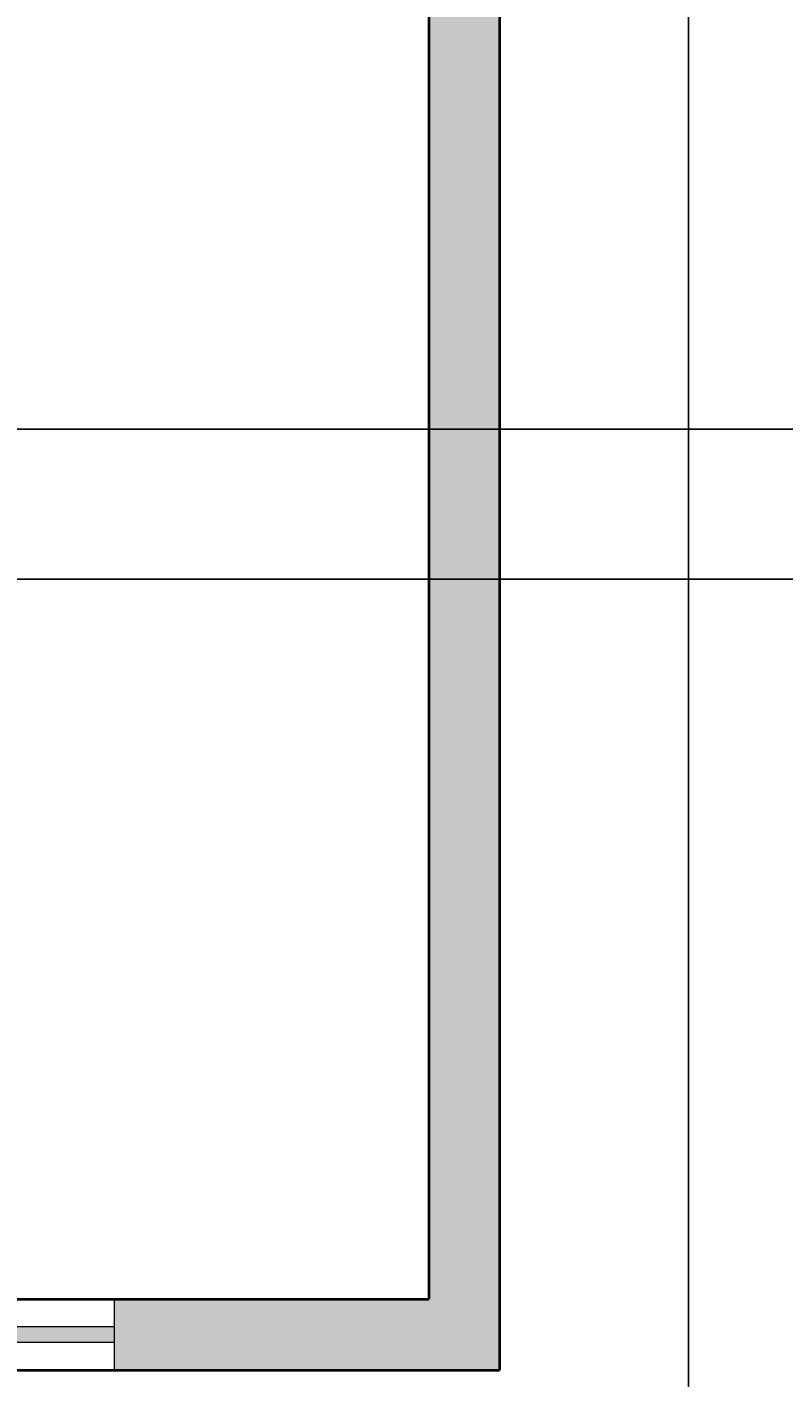
# Model space of a CAD drawing. Units: inches. Extents: x 2330 to 3943, y 1763 to 3461.
# Tile 8 of 40: x 2634 to 2730, y 2211 to 2383. Entities that reach past the tile are written whole.
import ezdxf

# ---------------------------------------------------------------- set-up
doc = ezdxf.new("R2010")
doc.units = ezdxf.units.IN
for name, color, linetype, lineweight in [('A-ANNO-DIMS', 2, 'Continuous', 18), ('A-GLAZ', 4, 'Continuous', 18), ('A-WALL', 7, 'Continuous', 40), ('A-WALL-PATT', 252, 'Continuous', 13)]:
    doc.layers.add(name, color=color, linetype=linetype, lineweight=lineweight)
doc.styles.get("Standard").update_dxf_attribs({"font": 'arial.ttf'})
doc.dimstyles.get("Standard").update_dxf_attribs({"dimtxt": 0.18, "dimasz": 0.18, "dimexe": 0.18, "dimexo": 0.0625, "dimgap": 0.09, "dimtad": 0, "dimtih": 1, "dimtoh": 1, "dimdec": 4, "dimzin": 0, "dimdsep": 46, "dimtxsty": 'Standard', "dimcen": 0.09, "dimadec": 0, "dimazin": 0, "dimtfac": 1, "dimtdec": 4, "dimtofl": 0, "dimtmove": 0, "dimatfit": 3, "dimfxl": 1, "dimtolj": 1, "dimtzin": 0, "dimarcsym": 0})

# ---------------------------------------------------------------- blocks, each defined once
blk = doc.blocks.new('WINDOW-120IN')
h = blk.add_hatch(color=256)
h.dxf.hatch_style = 1
h.paths.add_polyline_path([(120, 5.5), (0, 5.5), (0, 3.5), (120, 3.5)])
for p, q in [((0, 9), (0, 0)), ((120, 9), (120, 0)), ((120, 5.5), (0, 5.5)), ((120, 3.5), (0, 3.5))]:
    blk.add_line(p, q)
blk = doc.blocks.new('*D77')
at = {"layer": 'A-ANNO-DIMS', "color": 0, "lineweight": -2, "transparency": 16777216}
for p, q in [((2717.66, 2412.59), (2717.66, 1901.2)), ((2944.66, 2412.59), (2944.66, 1901.2)), ((2717.84, 1901.38), (2830.87, 1901.38)), ((2944.48, 1901.38), (2831.45, 1901.38))]:
    blk.add_line(p, q, dxfattribs=at)
at = {"layer": 'A-ANNO-DIMS', "color": 0, "transparency": 16777216}
for points in [[(2717.84, 1901.41), (2717.84, 1901.35), (2717.66, 1901.38)], [(2944.48, 1901.41), (2944.48, 1901.35), (2944.66, 1901.38)]]:
    blk.add_solid(points, dxfattribs=at)
at = {"layer": 'Defpoints', "color": 0, "transparency": 16777216}
for p in [(2717.66, 2412.65), (2944.66, 2412.65), (2944.66, 1901.38)]:
    blk.add_point(p, dxfattribs=at)
at = {"layer": 'A-ANNO-DIMS', "color": 0, "transparency": 16777216, "insert": (2831.16, 1901.38), "char_height": 0.18, "attachment_point": 5}
blk.add_mtext('\\A1;227', dxfattribs=at)
blk = doc.blocks.new('*D80')
at = {"layer": 'A-ANNO-DIMS', "color": 0, "lineweight": -2, "transparency": 16777216}
for p, q in [((3166.6, 2331.7), (2330.5, 2331.7)), ((2330.68, 2331.52), (2330.68, 2322.36)), ((2330.68, 2312.83), (2330.68, 2321.99)), ((3166.6, 2312.65), (2330.5, 2312.65))]:
    blk.add_line(p, q, dxfattribs=at)
at = {"layer": 'A-ANNO-DIMS', "color": 0, "transparency": 16777216}
for points in [[(2330.65, 2331.52), (2330.71, 2331.52), (2330.68, 2331.7)], [(2330.65, 2312.83), (2330.71, 2312.83), (2330.68, 2312.65)]]:
    blk.add_solid(points, dxfattribs=at)
at = {"layer": 'Defpoints', "color": 0, "transparency": 16777216}
for p in [(2330.68, 2331.7), (3166.66, 2331.7), (3166.66, 2312.65)]:
    blk.add_point(p, dxfattribs=at)
at = {"layer": 'A-ANNO-DIMS', "color": 0, "transparency": 16777216, "insert": (2330.68, 2322.18), "char_height": 0.18, "attachment_point": 5}
blk.add_mtext('\\A1;19.046', dxfattribs=at)

msp = doc.modelspace()

# ---------------------------------------------------------------- hatches: boundary and pattern name
at = {"layer": 'A-WALL-PATT'}
h = msp.add_hatch(color=256, dxfattribs=at)
h.dxf.hatch_style = 1
h.paths.add_polyline_path([(2693.6605, 2511.1524), (2684.6605, 2511.1524), (2684.6605, 2221.1524), (2644.6605, 2221.1524), (2644.6605, 2212.1524), (2693.6605, 2212.1524)])

# ---------------------------------------------------------------- linework, layer by layer
at = {"layer": 'A-WALL'}
for p, q in [((2684.6605, 2511.1524), (2684.6605, 2221.1524)), ((2693.6605, 2511.1524), (2693.6605, 2212.1524)), ((2484.6605, 2221.1524), (2684.6605, 2221.1524)), ((2475.6605, 2212.1524), (2693.6605, 2212.1524))]:
    msp.add_line(p, q, dxfattribs=at)

# ---------------------------------------------------------------- block references
at = {"layer": 'A-GLAZ'}
msp.add_blockref('WINDOW-120IN', (2524.6605, 2212.1524), dxfattribs=at)

# ---------------------------------------------------------------- dimensions: what is measured, and where the dimension line sits
at = {"layer": 'A-ANNO-DIMS'}
dim = msp.add_linear_dim(base=(2944.6605, 1901.3774), p1=(2717.6605, 2412.6524), p2=(2944.6605, 2412.6524), dimstyle='Standard', override={"dimdec": 0, "dimlfac": 1, "dimrnd": 0, "dimzin": 0, "dimdsep": 46, "dimlunit": 2}, dxfattribs=at)
dim.commit()
dim.dimension.update_dxf_attribs({"geometry": '*D77', "text_midpoint": (2831.1605, 1901.3774)})
dim = msp.add_linear_dim(base=(2330.6824, 2331.6982), p1=(3166.6605, 2312.6524), p2=(3166.6605, 2331.6982), angle=90, dimstyle='Standard', override={"dimdec": 3, "dimlfac": 1, "dimrnd": 0, "dimzin": 0, "dimdsep": 46, "dimlunit": 2}, dxfattribs=at)
dim.commit()
dim.dimension.update_dxf_attribs({"geometry": '*D80', "text_midpoint": (2330.6824, 2322.1753)})

doc.saveas('drawing.dxf')
